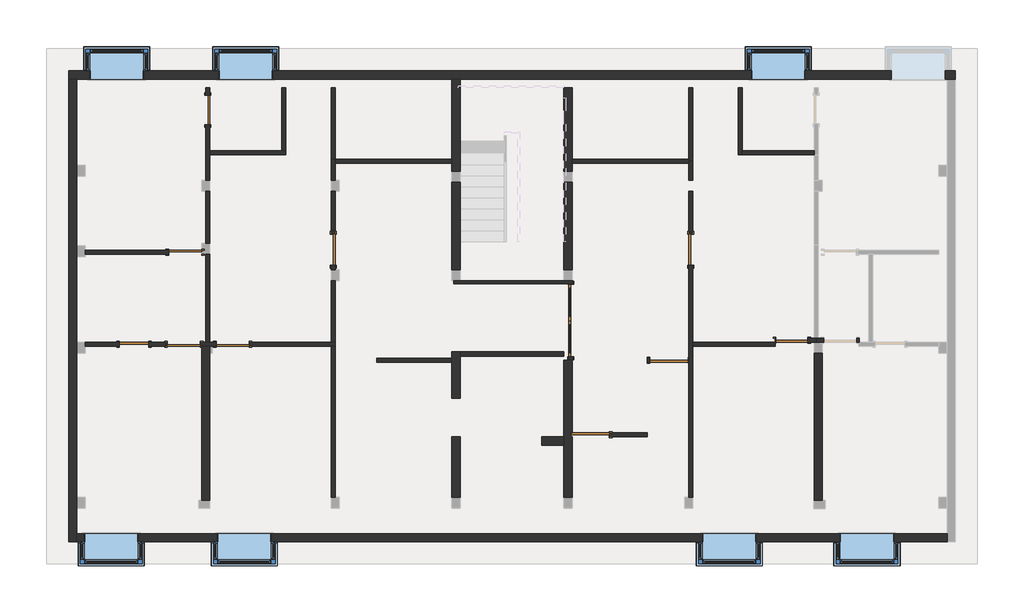
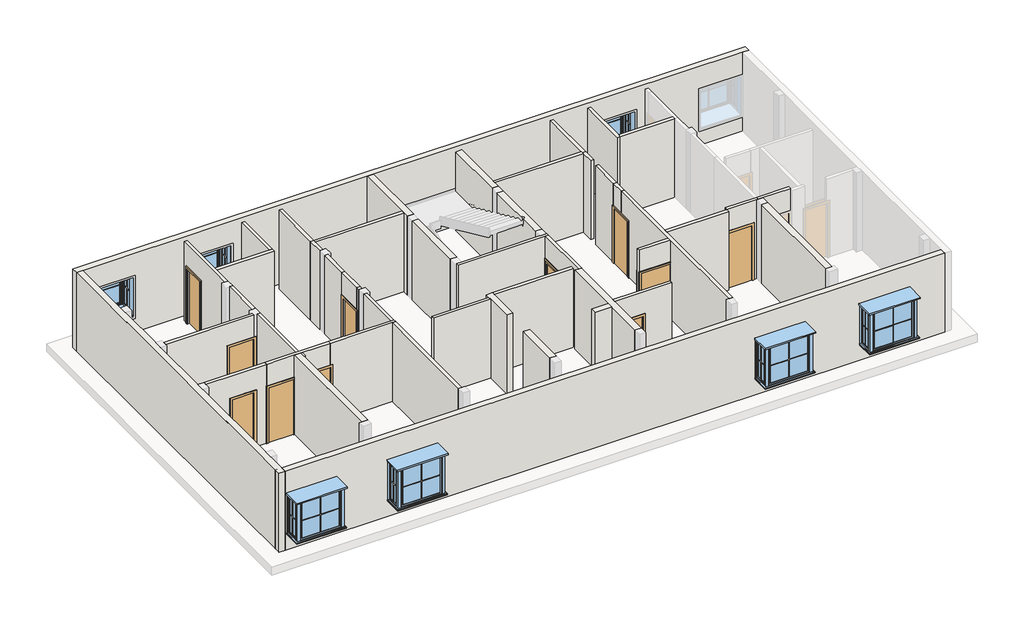
# One storey, part 1 of 2: 48 walls, 11 doors, 7 windows.
"""IFC4 building model written with IfcOpenShell, lengths in millimetres."""

from ifc_helpers import new_model, si_unit, frame, origin, place, context, project, spatial, polyline, outline, extrude, faceted_brep, transform, mapped, element, save
from components import door_04ab2522, m_door_single_panel_05506f71, door_07b5d71c, door_85b31ab1, door_1991e9a2, door_4c0a2014, door_82def9da, m_door_single_panel_3_x7_f8176753, m_door_single_panel_3_x7_ebb67e73, window_19bbd869

model = new_model("IFC4")

# Units and contexts
model_context = context("Model", 3, world=origin())
ifc_project = project(units=[si_unit("LENGTHUNIT", "METRE", prefix="MILLI")], contexts=[model_context])

# Site, building, storey
site = spatial("IfcSite", under=ifc_project)
building = spatial("IfcBuilding", under=site)
storey = spatial("IfcBuildingStorey", under=building, Elevation=16002.0)

# Doors
placement = place(None, origin())
door_shape = door_04ab2522(model_context)
element("IfcDoor", 1, ObjectType="M_Door-Double-Glass : 6'7\"X7'", at=placement, inside=storey, context=model_context, shape_type="MappedRepresentation", body=[
    mapped(door_shape, transform((1217.5394962, 1183.3817656, 16002.0), x_axis=(0.0, 1.0, 0.0), y_axis=(-1.0, 0.0, 0.0), z_axis=(0.0, 0.0, 1.0))),
])
m_door_single_panel_shape = m_door_single_panel_05506f71(model_context)
element("IfcDoor", 2, ObjectType="M_Door-Single-Panel", at=placement, inside=storey, context=model_context, shape_type="MappedRepresentation", body=[
    mapped(m_door_single_panel_shape, transform((1745.3012085, -1975.7432663, 16002.0), x_axis=(-1.0, 0.0, 0.0), y_axis=(0.0, -1.0, 0.0), z_axis=(0.0, 0.0, 1.0))),
])
element("IfcDoor", 3, ObjectType="M_Door-Single-Panel", at=placement, inside=storey, context=model_context, shape_type="MappedRepresentation", body=[
    mapped(m_door_single_panel_shape, transform((3933.4813133, 90.9578621, 16002.0), x_axis=(1.0, 0.0, 0.0), y_axis=(0.0, 1.0, 0.0), z_axis=(0.0, 0.0, 1.0))),
])
door_2_shape = door_07b5d71c(model_context)
element("IfcDoor", 4, ObjectType="M_Door-Single-Panel : 2'10\"X7' 2", at=placement, inside=storey, context=model_context, shape_type="MappedRepresentation", body=[
    mapped(door_2_shape, transform((-5360.3487995, 3142.9626891, 16002.0), x_axis=(0.0, -1.0, 0.0), y_axis=(1.0, 0.0, 0.0), z_axis=(0.0, 0.0, 1.0))),
])
door_3_shape = door_85b31ab1(model_context)
element("IfcDoor", 5, ObjectType="M_Door-Single-Panel : 2'10\"X7' 2", at=placement, inside=storey, context=model_context, shape_type="MappedRepresentation", body=[
    mapped(door_3_shape, transform((4532.9512082, 3142.9626891, 16002.0), x_axis=(0.0, -1.0, 0.0), y_axis=(1.0, 0.0, 0.0), z_axis=(0.0, 0.0, 1.0))),
])
door_4_shape = door_1991e9a2(model_context)
element("IfcDoor", 6, ObjectType="M_Door-Single-Panel : 2'11\"X7' 3", at=placement, inside=storey, context=model_context, shape_type="MappedRepresentation", body=[
    mapped(door_4_shape, transform((7330.1405552, 640.4567334, 16002.0), x_axis=(1.0, 0.0, 0.0), y_axis=(0.0, 1.0, 0.0), z_axis=(0.0, 0.0, 1.0))),
])
door_5_shape = door_4c0a2014(model_context)
element("IfcDoor", 7, ObjectType="M_Door-Single-Panel : 2'8\"X7'", at=placement, inside=storey, context=model_context, shape_type="MappedRepresentation", body=[
    mapped(door_5_shape, transform((-10873.4462614, 526.1567334, 16002.0), x_axis=(1.0, 0.0, 0.0), y_axis=(0.0, 1.0, 0.0), z_axis=(0.0, 0.0, 1.0))),
])
door_6_shape = door_82def9da(model_context)
element("IfcDoor", 8, ObjectType="M_Door-Single-Panel : 2'8\"X7'", at=placement, inside=storey, context=model_context, shape_type="MappedRepresentation", body=[
    mapped(door_6_shape, transform((-8827.4487992, 7008.6751452, 16002.0), x_axis=(0.0, 1.0, 0.0), y_axis=(-1.0, 0.0, 0.0), z_axis=(0.0, 0.0, 1.0))),
])
m_door_single_panel_3_x7_shape = m_door_single_panel_3_x7_f8176753(model_context)
element("IfcDoor", 9, ObjectType="M_Door-Single-Panel : 3'X7'", at=placement, inside=storey, context=model_context, shape_type="MappedRepresentation", body=[
    mapped(m_door_single_panel_3_x7_shape, transform((-9456.0987989, 3078.8567332, 16002.0), x_axis=(1.0, 0.0, 0.0), y_axis=(0.0, 1.0, 0.0), z_axis=(0.0, 0.0, 1.0))),
])
element("IfcDoor", 10, ObjectType="M_Door-Single-Panel : 3'X7'", at=placement, inside=storey, context=model_context, shape_type="MappedRepresentation", body=[
    mapped(m_door_single_panel_3_x7_shape, transform((-8144.8381465, 526.1567334, 16002.0), x_axis=(-1.0, 0.0, 0.0), y_axis=(0.0, -1.0, 0.0), z_axis=(0.0, 0.0, 1.0))),
])
m_door_single_panel_3_x7_2_shape = m_door_single_panel_3_x7_ebb67e73(model_context)
element("IfcDoor", 11, ObjectType="M_Door-Single-Panel : 3'X7'", at=placement, inside=storey, context=model_context, shape_type="MappedRepresentation", body=[
    mapped(m_door_single_panel_3_x7_2_shape, transform((-9494.1987992, 526.1567334, 16002.0), x_axis=(1.0, 0.0, 0.0), y_axis=(0.0, 1.0, 0.0), z_axis=(0.0, 0.0, 1.0))),
])

# Walls
element("IfcWall", 12, ObjectType="3.5\"", at=placement, inside=storey, context=model_context, shape_type="Brep", body=[
    faceted_brep([(-2020.2487998, 2196.2067742, 16002.0), (1158.0082462, 2196.2067742, 16002.0), (1272.3082462, 2196.2067742, 16002.0), (1272.3082462, 2196.2067742, 19050.0), (1158.0082462, 2196.2067742, 19050.0), (-2020.2487998, 2196.2067742, 19050.0), (-2020.2487998, 2285.1067742, 16002.0), (-2020.2487998, 2285.1067742, 19050.0), (-1845.5417538, 2285.1067742, 19050.0), (1024.6582462, 2285.1067742, 19050.0), (1253.2582462, 2285.1067742, 19050.0), (1272.3082462, 2285.1067742, 19050.0), (1272.3082462, 2285.1067742, 16002.0), (1253.2582462, 2285.1067742, 16002.0), (1024.6582462, 2285.1067742, 16002.0), (-1845.5417538, 2285.1067742, 16002.0)], [[[0, 1, 2, 3, 4, 5]], [[6, 7, 8, 9, 10, 11, 12, 13, 14, 15]], [[2, 1, 0, 6, 15, 14, 13, 12]], [[5, 4, 3, 11, 10, 9, 8, 7]], [[0, 5, 7, 6]], [[3, 2, 12, 11]]]),
])
element("IfcWall", 13, ObjectType="4.5\"", at=placement, inside=storey, context=model_context, shape_type="SweptSolid", body=[
    extrude(outline(polyline([(3132.0737955, 19050.0), (3628.3344162, 19050.0), (3628.3344162, 16002.0), (3574.7626891, 16002.0), (3574.7626891, 18135.6), (3132.0737955, 18135.6), (3132.0737955, 19050.0)])), frame((4475.8012082, 0.0, 0.0), z_axis=(1.0, 0.0, 0.0), x_axis=(0.0, 1.0, 0.0)), (0.0, 0.0, 1.0), 114.3),
])
element("IfcWall", 14, ObjectType="4.5\"", at=placement, inside=storey, context=model_context, shape_type="SweptSolid", body=[
    extrude(outline(polyline([(2711.1626891, 19050.0), (3671.8272228, 19050.0), (3671.8272228, 16002.0), (3574.7626891, 16002.0), (3574.7626891, 18135.6), (2711.1626891, 18135.6), (2711.1626891, 19050.0)])), frame((-5417.4987995, 0.0, 0.0), z_axis=(1.0, 0.0, 0.0), x_axis=(0.0, 1.0, 0.0)), (0.0, 0.0, 1.0), 114.3),
])
element("IfcWall", 15, ObjectType="4.5\"", at=placement, inside=storey, context=model_context, shape_type="Brep", body=[
    faceted_brep([(-7690.1644155, 469.0067334, 19050.0), (-8713.148796, 469.0067334, 19050.0), (-8771.750543, 469.0067334, 19050.0), (-9000.350543, 469.0067334, 19050.0), (-10009.8462614, 469.0067334, 19050.0), (-10009.8462614, 469.0067334, 16002.0), (-9951.3987992, 469.0067334, 16002.0), (-9951.3987992, 469.0067334, 18135.6), (-9036.9987992, 469.0067334, 18135.6), (-9036.9987992, 469.0067334, 16002.0), (-9000.350543, 469.0067334, 16002.0), (-8771.750543, 469.0067334, 16002.0), (-8713.148796, 469.0067334, 16002.0), (-8602.0381465, 469.0067334, 16002.0), (-8602.0381465, 469.0067334, 18135.6), (-7690.1644155, 469.0067334, 18135.6), (-10009.8462614, 583.3067334, 19050.0), (-7690.1644155, 583.3067334, 19050.0), (-7690.1644155, 583.3067334, 18135.6), (-8602.0381465, 583.3067334, 18135.6), (-8602.0381465, 583.3067334, 16002.0), (-9036.9987992, 583.3067334, 16002.0), (-9036.9987992, 583.3067334, 18135.6), (-9951.3987992, 583.3067334, 18135.6), (-9951.3987992, 583.3067334, 16002.0), (-10009.8462614, 583.3067334, 16002.0)], [[[0, 1, 2, 3, 4, 5, 6, 7, 8, 9, 10, 11, 12, 13, 14, 15]], [[16, 17, 18, 19, 20, 21, 22, 23, 24, 25]], [[5, 25, 24, 6]], [[9, 21, 20, 13, 12, 11, 10]], [[17, 0, 15, 18]], [[4, 3, 2, 1, 0, 17, 16]], [[5, 4, 16, 25]], [[8, 22, 21, 9]], [[7, 23, 22, 8]], [[23, 7, 6, 24]], [[19, 14, 13, 20]], [[14, 19, 18, 15]]]),
])
element("IfcWall", 16, ObjectType="4.5\"", at=placement, inside=storey, context=model_context, shape_type="Brep", body=[
    faceted_brep([(8000.0512079, 583.3067334, 16002.0), (8000.0512079, 583.3067334, 19050.0), (7942.9012047, 583.3067334, 19050.0), (6862.7668241, 583.3067334, 19050.0), (6862.7668241, 583.3067334, 16002.0), (6885.6405552, 583.3067334, 16002.0), (6885.6405552, 583.3067334, 18135.6), (7774.6405552, 583.3067334, 18135.6), (7774.6405552, 583.3067334, 16002.0), (7942.9012047, 583.3067334, 16002.0), (8000.0512079, 697.6067334, 19050.0), (8000.0512079, 697.6067334, 16002.0), (7942.9012079, 697.6067334, 16002.0), (7774.6405552, 697.6067334, 16002.0), (7774.6405552, 697.6067334, 18135.6), (6885.6405552, 697.6067334, 18135.6), (6885.6405552, 697.6067334, 16002.0), (6862.7668241, 697.6067334, 16002.0), (6862.7668241, 697.6067334, 19050.0), (7942.9012079, 697.6067334, 19050.0)], [[[0, 1, 2, 3, 4, 5, 6, 7, 8, 9]], [[10, 11, 12, 13, 14, 15, 16, 17, 18, 19]], [[4, 17, 16, 5]], [[11, 0, 9, 8, 13, 12]], [[1, 0, 11, 10]], [[3, 2, 1, 10, 19, 18]], [[4, 3, 18, 17]], [[7, 14, 13, 8]], [[14, 7, 6, 15]], [[15, 6, 5, 16]]]),
])
element("IfcWall", 17, ObjectType="4.5\"", at=placement, inside=storey, context=model_context, shape_type="Brep", body=[
    faceted_brep([(9187.5012047, 583.3067334, 16002.0), (9187.5012047, 583.3067334, 19050.0), (8171.5012047, 583.3067334, 19050.0), (8000.0512079, 583.3067334, 19050.0), (8000.0512079, 583.3067334, 16002.0), (8171.5012047, 583.3067334, 16002.0), (8209.6012079, 583.3067334, 16002.0), (8209.6012079, 583.3067334, 18135.6), (9124.0012079, 583.3067334, 18135.6), (9124.0012079, 583.3067334, 16002.0), (9187.5012047, 697.6067334, 19050.0), (9187.5012047, 697.6067334, 16002.0), (9124.0012079, 697.6067334, 16002.0), (9124.0012079, 697.6067334, 18135.6), (8209.6012079, 697.6067334, 18135.6), (8209.6012079, 697.6067334, 16002.0), (8057.2012079, 697.6067334, 16002.0), (8000.0512079, 697.6067334, 16002.0), (8000.0512079, 697.6067334, 19050.0), (8057.2012079, 697.6067334, 19050.0)], [[[0, 1, 2, 3, 4, 5, 6, 7, 8, 9]], [[10, 11, 12, 13, 14, 15, 16, 17, 18, 19]], [[11, 0, 9, 12]], [[4, 17, 16, 15, 6, 5]], [[1, 0, 11, 10]], [[3, 2, 1, 10, 19, 18]], [[4, 3, 18, 17]], [[7, 14, 13, 8]], [[8, 13, 12, 9]], [[14, 7, 6, 15]]]),
])
element("IfcWall", 18, ObjectType="4.5\"", at=placement, inside=storey, context=model_context, shape_type="SweptSolid", body=[
    extrude(outline(polyline([(16002.0, 3334.0114184), (19050.0, 3334.0114184), (19050.0, 1250.0012085), (18135.6, 1250.0012085), (18135.6, 2278.7012085), (16002.0, 2278.7012085), (16002.0, 3334.0114184)])), frame((0.0, -2032.8932663, 0.0), z_axis=(0.0, 1.0, 0.0), x_axis=(0.0, 0.0, 1.0)), (0.0, 0.0, 1.0), 114.3),
])
element("IfcWall", 19, ObjectType="4.5\"", at=placement, inside=storey, context=model_context, shape_type="SweptSolid", body=[
    extrude(outline(polyline([(18135.6, 4466.8813133), (16002.0, 4466.8813133), (16002.0, 4475.8012082), (19050.0, 4475.8012082), (19050.0, 3334.0114184), (16002.0, 3334.0114184), (16002.0, 3400.0813133), (18135.6, 3400.0813133), (18135.6, 4466.8813133)])), frame((0.0, 33.8078621, 0.0), z_axis=(0.0, 1.0, 0.0), x_axis=(0.0, 0.0, 1.0)), (0.0, 0.0, 1.0), 114.3),
])
element("IfcWall", 20, ObjectType="4.5\"", at=placement, inside=storey, context=model_context, shape_type="SweptSolid", body=[
    extrude(outline(polyline([(1021.4012085, 202.3067742), (-1848.7987998, 202.3067742), (-1848.7987998, 316.6067742), (1021.4012085, 316.6067742), (1021.4012085, 202.3067742)])), frame((0.0, 0.0, 16002.0), z_axis=(0.0, 0.0, 1.0), x_axis=(1.0, 0.0, 0.0)), (0.0, 0.0, 1.0), 3048.0),
])
element("IfcWall", 21, ObjectType="4.5\"", at=placement, inside=storey, context=model_context, shape_type="Brep", body=[
    faceted_brep([(1158.0082462, 2196.2067742, 16002.0), (1158.0082462, 2186.6817656, 16002.0), (1158.0082462, 2186.6817656, 18135.6), (1158.0082462, 180.0817656, 18135.6), (1158.0082462, 180.0817656, 16002.0), (1158.0082462, 90.9578621, 16002.0), (1158.0082462, 90.9578621, 19050.0), (1158.0082462, 2196.2067742, 19050.0), (1272.3082462, 2186.6817656, 18135.6), (1272.3082462, 2186.6817656, 16002.0), (1272.3082462, 2196.2067742, 16002.0), (1272.3082462, 2196.2067742, 19050.0), (1272.3082462, 90.9578621, 19050.0), (1272.3082462, 90.9578621, 16002.0), (1272.3082462, 180.0817656, 16002.0), (1272.3082462, 180.0817656, 18135.6), (1250.0012085, 90.9578621, 16002.0), (1250.0012085, 90.9578621, 19050.0)], [[[0, 1, 2, 3, 4, 5, 6, 7]], [[8, 9, 10, 11, 12, 13, 14, 15]], [[14, 13, 16, 5, 4]], [[10, 9, 1, 0]], [[6, 5, 16, 13, 12, 17]], [[7, 6, 17, 12, 11]], [[0, 7, 11, 10]], [[2, 1, 9, 8]], [[3, 2, 8, 15]], [[4, 3, 15, 14]]]),
])
element("IfcWall", 22, ObjectType="4.5\"", at=placement, inside=storey, context=model_context, shape_type="Brep", body=[
    faceted_brep([(1250.0012085, 5536.3067329, 16002.0), (4475.8012082, 5536.3067329, 16002.0), (4475.8012082, 5536.3067329, 19050.0), (1250.0012085, 5536.3067329, 19050.0), (1250.0012085, 5650.6067329, 16002.0), (1250.0012085, 5650.6067329, 19050.0), (4475.8012082, 5650.6067329, 19050.0), (4475.8012082, 5650.6067329, 16002.0), (4475.8012082, 5593.4567329, 16002.0), (4475.8012082, 5593.4567329, 19050.0)], [[[0, 1, 2, 3]], [[4, 5, 6, 7]], [[1, 0, 4, 7, 8]], [[3, 2, 9, 6, 5]], [[2, 1, 8, 7, 6, 9]], [[0, 3, 5, 4]]]),
])
element("IfcWall", 23, ObjectType="4.5\"", at=placement, inside=storey, context=model_context, shape_type="SweptSolid", body=[
    extrude(outline(polyline([(-5417.4987995, -3709.2932193), (-5417.4987995, 469.0067334), (-5303.1987995, 469.0067334), (-5303.1987995, -3709.2932193), (-5417.4987995, -3709.2932193)])), frame((0.0, 0.0, 16002.0), z_axis=(0.0, 0.0, 1.0), x_axis=(1.0, 0.0, 0.0)), (0.0, 0.0, 1.0), 3048.0),
])
element("IfcWall", 24, ObjectType="4.5\" 2", at=placement, inside=storey, context=model_context, shape_type="SweptSolid", body=[
    extrude(outline(polyline([(19050.0, -8998.8987989), (19050.0, -12224.6987989), (16002.0, -12224.6987989), (16002.0, -9913.2987989), (18135.6, -9913.2987989), (18135.6, -8998.8987989), (19050.0, -8998.8987989)])), frame((0.0, 3021.7067332, 0.0), z_axis=(0.0, 1.0, 0.0), x_axis=(0.0, 0.0, 1.0)), (0.0, 0.0, 1.0), 114.3),
])
element("IfcWall", 25, ObjectType="4.5\" 2", at=placement, inside=storey, context=model_context, shape_type="SweptSolid", body=[
    extrude(outline(polyline([(-8770.2987992, 4761.606733), (-8770.2987992, 3326.5067332), (-8884.5987992, 3326.5067332), (-8884.5987992, 4761.606733), (-8770.2987992, 4761.606733)])), frame((0.0, 0.0, 16002.0), z_axis=(0.0, 0.0, 1.0), x_axis=(1.0, 0.0, 0.0)), (0.0, 0.0, 1.0), 3048.0),
])
element("IfcWall", 26, ObjectType="4.5\" 2", at=placement, inside=storey, context=model_context, shape_type="Brep", body=[
    faceted_brep([(-8770.2987992, 7415.0751452, 18135.6), (-8770.2987992, 7415.0751452, 16002.0), (-8770.2987992, 7631.8067329, 16002.0), (-8770.2987992, 7631.8067329, 19050.0), (-8770.2987992, 5879.2067329, 19050.0), (-8770.2987992, 5764.9067329, 19050.0), (-8770.2987992, 5066.406733, 19050.0), (-8770.2987992, 5066.406733, 16002.0), (-8770.2987992, 5764.9067329, 16002.0), (-8770.2987992, 5879.2067329, 16002.0), (-8770.2987992, 6602.2751452, 16002.0), (-8770.2987992, 6602.2751452, 18135.6), (-8884.5987992, 7631.8067329, 16002.0), (-8884.5987992, 7415.0751452, 16002.0), (-8884.5987992, 7415.0751452, 18135.6), (-8884.5987992, 6602.2751452, 18135.6), (-8884.5987992, 6602.2751452, 16002.0), (-8884.5987992, 5066.406733, 16002.0), (-8884.5987992, 5066.406733, 19050.0), (-8884.5987992, 7631.8067329, 19050.0)], [[[0, 1, 2, 3, 4, 5, 6, 7, 8, 9, 10, 11]], [[12, 13, 14, 15, 16, 17, 18, 19]], [[2, 1, 13, 12]], [[10, 9, 8, 7, 17, 16]], [[3, 2, 12, 19]], [[6, 5, 4, 3, 19, 18]], [[7, 6, 18, 17]], [[14, 13, 1, 0]], [[15, 14, 0, 11]], [[16, 15, 11, 10]]]),
])
element("IfcWall", 27, ObjectType="4.5\" 2", at=placement, inside=storey, context=model_context, shape_type="Brep", body=[
    faceted_brep([(-8770.2987992, 5764.9067329, 16002.0), (-6674.7987994, 5764.9067329, 16002.0), (-6674.7987994, 5764.9067329, 19050.0), (-8770.2987992, 5764.9067329, 19050.0), (-8770.2987992, 5879.2067329, 16002.0), (-8770.2987992, 5879.2067329, 19050.0), (-6789.0987994, 5879.2067329, 19050.0), (-6674.7987994, 5879.2067329, 19050.0), (-6674.7987994, 5879.2067329, 16002.0), (-6789.0987994, 5879.2067329, 16002.0)], [[[0, 1, 2, 3]], [[4, 5, 6, 7, 8, 9]], [[1, 0, 4, 9, 8]], [[3, 2, 7, 6, 5]], [[0, 3, 5, 4]], [[2, 1, 8, 7]]]),
])
element("IfcWall", 28, ObjectType="4.5\" 2", at=placement, inside=storey, context=model_context, shape_type="SweptSolid", body=[
    extrude(outline(polyline([(-6674.7987994, 7631.8067329), (-6674.7987994, 5879.2067329), (-6789.0987994, 5879.2067329), (-6789.0987994, 7631.8067329), (-6674.7987994, 7631.8067329)])), frame((0.0, 0.0, 16002.0), z_axis=(0.0, 0.0, 1.0), x_axis=(1.0, 0.0, 0.0)), (0.0, 0.0, 1.0), 3048.0),
])
element("IfcWall", 29, ObjectType="4.5\" 2", at=placement, inside=storey, context=model_context, shape_type="SweptSolid", body=[
    extrude(outline(polyline([(18135.6, -10467.0462614), (16002.0, -10467.0462614), (16002.0, -10009.8462614), (19050.0, -10009.8462614), (19050.0, -12224.6987989), (16002.0, -12224.6987989), (16002.0, -11279.8462614), (18135.6, -11279.8462614), (18135.6, -10467.0462614)])), frame((0.0, 469.0067334, 0.0), z_axis=(0.0, 1.0, 0.0), x_axis=(0.0, 0.0, 1.0)), (0.0, 0.0, 1.0), 114.3),
])
element("IfcWall", 30, ObjectType="4.5\" 2", at=placement, inside=storey, context=model_context, shape_type="SweptSolid", body=[
    extrude(outline(polyline([(-8770.298796, 3021.7067332), (-8770.298796, 583.3067804), (-8884.598796, 583.3067804), (-8884.598796, 3021.7067332), (-8770.298796, 3021.7067332)])), frame((0.0, 0.0, 16002.0), z_axis=(0.0, 0.0, 1.0), x_axis=(1.0, 0.0, 0.0)), (0.0, 0.0, 1.0), 3048.0),
])
element("IfcWall", 31, ObjectType="4.5\" 2", at=placement, inside=storey, context=model_context, shape_type="Brep", body=[
    faceted_brep([(-5303.1987995, 469.0067334, 19050.0), (-5417.4987995, 469.0067334, 19050.0), (-7690.1644155, 469.0067334, 19050.0), (-7690.1644155, 469.0067334, 18135.6), (-7687.6381465, 469.0067334, 18135.6), (-7687.6381465, 469.0067334, 16002.0), (-5417.4987995, 469.0067334, 16002.0), (-5303.1987995, 469.0067334, 16002.0), (-7690.1644155, 583.3067334, 19050.0), (-5417.4987995, 583.3067334, 19050.0), (-5303.1987995, 583.3067334, 19050.0), (-5303.1987995, 583.3067334, 16002.0), (-5417.4987995, 583.3067334, 16002.0), (-7687.6381465, 583.3067334, 16002.0), (-7687.6381465, 583.3067334, 18135.6), (-7690.1644155, 583.3067334, 18135.6)], [[[0, 1, 2, 3, 4, 5, 6, 7]], [[8, 9, 10, 11, 12, 13, 14, 15]], [[11, 7, 6, 5, 13, 12]], [[2, 1, 0, 10, 9, 8]], [[2, 8, 15, 3]], [[0, 7, 11, 10]], [[14, 4, 3, 15]], [[4, 14, 13, 5]]]),
])
element("IfcWall", 32, ObjectType="4.5\" 2", at=placement, inside=storey, context=model_context, shape_type="SweptSolid", body=[
    extrude(outline(polyline([(-5303.1987995, 2285.1067802), (-5303.1987995, 583.3067334), (-5417.4987995, 583.3067334), (-5417.4987995, 2285.1067802), (-5303.1987995, 2285.1067802)])), frame((0.0, 0.0, 16002.0), z_axis=(0.0, 0.0, 1.0), x_axis=(1.0, 0.0, 0.0)), (0.0, 0.0, 1.0), 3048.0),
])
element("IfcWall", 33, ObjectType="4.5\" 2", at=placement, inside=storey, context=model_context, shape_type="Brep", body=[
    faceted_brep([(-5303.1987995, 2589.9067802, 16002.0), (-5303.1987995, 2711.1626891, 16002.0), (-5303.1987995, 2711.1626891, 18135.6), (-5303.1987995, 2711.1626891, 19050.0), (-5303.1987995, 2589.9067802, 19050.0), (-5417.4987995, 2589.9067802, 16002.0), (-5417.4987995, 2589.9067802, 19050.0), (-5417.4987995, 2711.1626891, 19050.0), (-5417.4987995, 2711.1626891, 18135.6), (-5417.4987995, 2711.1626891, 16002.0)], [[[0, 1, 2, 3, 4]], [[5, 6, 7, 8, 9]], [[1, 0, 5, 9]], [[3, 2, 1, 9, 8, 7]], [[4, 3, 7, 6]], [[0, 4, 6, 5]]]),
])
element("IfcWall", 34, ObjectType="4.5\" 2", at=placement, inside=storey, context=model_context, shape_type="SweptSolid", body=[
    extrude(outline(polyline([(-5303.1987995, 4761.606733), (-5303.1987995, 3671.8272228), (-5417.4987995, 3671.8272228), (-5417.4987995, 4761.606733), (-5303.1987995, 4761.606733)])), frame((0.0, 0.0, 16002.0), z_axis=(0.0, 0.0, 1.0), x_axis=(1.0, 0.0, 0.0)), (0.0, 0.0, 1.0), 3048.0),
])
element("IfcWall", 35, ObjectType="4.5\" 2", at=placement, inside=storey, context=model_context, shape_type="Brep", body=[
    faceted_brep([(-5303.1987995, 5066.406733, 16002.0), (-5303.1987995, 5536.3067329, 16002.0), (-5303.1987995, 5650.6067329, 16002.0), (-5303.1987995, 5650.6067329, 19050.0), (-5303.1987995, 5536.3067329, 19050.0), (-5303.1987995, 5066.406733, 19050.0), (-5417.4987995, 5066.406733, 16002.0), (-5417.4987995, 5066.406733, 19050.0), (-5417.4987995, 5650.6067329, 19050.0), (-5417.4987995, 5650.6067329, 16002.0)], [[[0, 1, 2, 3, 4, 5]], [[6, 7, 8, 9]], [[2, 1, 0, 6, 9]], [[5, 4, 3, 8, 7]], [[0, 5, 7, 6]], [[3, 2, 9, 8]]]),
])
element("IfcWall", 36, ObjectType="4.5\" 2", at=placement, inside=storey, context=model_context, shape_type="SweptSolid", body=[
    extrude(outline(polyline([(-2077.3987998, 5536.3067329), (-5303.1987995, 5536.3067329), (-5303.1987995, 5650.6067329), (-2077.3987998, 5650.6067329), (-2077.3987998, 5536.3067329)])), frame((0.0, 0.0, 16002.0), z_axis=(0.0, 0.0, 1.0), x_axis=(1.0, 0.0, 0.0)), (0.0, 0.0, 1.0), 3048.0),
])
element("IfcWall", 37, ObjectType="4.5\" 2", at=placement, inside=storey, context=model_context, shape_type="SweptSolid", body=[
    extrude(outline(polyline([(-5417.4987995, 5650.6067329), (-5417.4987995, 7631.8067329), (-5303.1987995, 7631.8067329), (-5303.1987995, 5650.6067329), (-5417.4987995, 5650.6067329)])), frame((0.0, 0.0, 16002.0), z_axis=(0.0, 0.0, 1.0), x_axis=(1.0, 0.0, 0.0)), (0.0, 0.0, 1.0), 3048.0),
])
element("IfcWall", 38, ObjectType="4.5\" 2", at=placement, inside=storey, context=model_context, shape_type="Brep", body=[
    faceted_brep([(4475.8012082, 5593.4567329, 16002.0), (4475.8012082, 5536.3067329, 16002.0), (4475.8012082, 5066.40678, 16002.0), (4475.8012082, 5066.40678, 19050.0), (4475.8012082, 5536.3067329, 19050.0), (4475.8012082, 5593.4567329, 19050.0), (4590.1012082, 5593.4567329, 16002.0), (4590.1012082, 5593.4567329, 19050.0), (4590.1012082, 5066.40678, 19050.0), (4590.1012082, 5066.40678, 16002.0)], [[[0, 1, 2, 3, 4, 5]], [[6, 7, 8, 9]], [[2, 1, 0, 6, 9]], [[3, 2, 9, 8]], [[5, 4, 3, 8, 7]], [[0, 5, 7, 6]]]),
])
element("IfcWall", 39, ObjectType="4.5\" 2", at=placement, inside=storey, context=model_context, shape_type="SweptSolid", body=[
    extrude(outline(polyline([(4475.8012082, 3628.3344162), (4475.8012082, 4761.606733), (4590.1012082, 4761.606733), (4590.1012082, 3628.3344162), (4475.8012082, 3628.3344162)])), frame((0.0, 0.0, 16002.0), z_axis=(0.0, 0.0, 1.0), x_axis=(1.0, 0.0, 0.0)), (0.0, 0.0, 1.0), 3048.0),
])
element("IfcWall", 40, ObjectType="4.5\" 2", at=placement, inside=storey, context=model_context, shape_type="Brep", body=[
    faceted_brep([(4475.8012082, -3709.2932193, 16002.0), (4475.8012082, -3709.2932193, 19050.0), (4475.8012082, 33.8078621, 19050.0), (4475.8012082, 148.1078621, 19050.0), (4475.8012082, 3132.0737955, 19050.0), (4475.8012082, 3132.0737955, 18135.6), (4475.8012082, 2711.1626891, 18135.6), (4475.8012082, 2711.1626891, 16002.0), (4475.8012082, 148.1078621, 16002.0), (4475.8012082, 33.8078621, 16002.0), (4590.1012082, -3709.2932193, 19050.0), (4590.1012082, -3709.2932193, 16002.0), (4590.1012082, 469.0067334, 16002.0), (4590.1012082, 583.3067334, 16002.0), (4590.1012082, 2711.1626891, 16002.0), (4590.1012082, 2711.1626891, 18135.6), (4590.1012082, 3132.0737955, 18135.6), (4590.1012082, 3132.0737955, 19050.0), (4590.1012082, 583.3067334, 19050.0), (4590.1012082, 469.0067334, 19050.0)], [[[0, 1, 2, 3, 4, 5, 6, 7, 8, 9]], [[10, 11, 12, 13, 14, 15, 16, 17, 18, 19]], [[11, 0, 9, 8, 7, 14, 13, 12]], [[1, 0, 11, 10]], [[4, 3, 2, 1, 10, 19, 18, 17]], [[4, 17, 16, 5]], [[6, 15, 14, 7]], [[15, 6, 5, 16]]]),
])
element("IfcWall", 41, ObjectType="4.5\" 2", at=placement, inside=storey, context=model_context, shape_type="SweptSolid", body=[
    extrude(outline(polyline([(6862.7668241, 469.0067334), (4590.1012082, 469.0067334), (4590.1012082, 583.3067334), (6862.7668241, 583.3067334), (6862.7668241, 469.0067334)])), frame((0.0, 0.0, 16002.0), z_axis=(0.0, 0.0, 1.0), x_axis=(1.0, 0.0, 0.0)), (0.0, 0.0, 1.0), 3048.0),
])
element("IfcWall", 42, ObjectType="4.5\" 2", at=placement, inside=storey, context=model_context, shape_type="Brep", body=[
    faceted_brep([(4590.1012082, 5593.4567329, 16002.0), (4590.1012082, 7631.8067329, 16002.0), (4590.1012082, 7631.8067329, 19050.0), (4590.1012082, 5593.4567329, 19050.0), (4475.8012082, 5593.4567329, 16002.0), (4475.8012082, 5593.4567329, 19050.0), (4475.8012082, 5650.6067329, 19050.0), (4475.8012082, 7631.8067329, 19050.0), (4475.8012082, 7631.8067329, 16002.0), (4475.8012082, 5650.6067329, 16002.0)], [[[0, 1, 2, 3]], [[4, 5, 6, 7, 8, 9]], [[1, 0, 4, 9, 8]], [[2, 1, 8, 7]], [[3, 2, 7, 6, 5]], [[0, 3, 5, 4]]]),
])
element("IfcWall", 43, ObjectType="4.5\" 2", at=placement, inside=storey, context=model_context, shape_type="Brep", body=[
    faceted_brep([(5847.401208, 7631.8067329, 16002.0), (5847.401208, 5764.9067329, 16002.0), (5847.401208, 5764.9067329, 19050.0), (5847.401208, 7631.8067329, 19050.0), (5961.701208, 7631.8067329, 16002.0), (5961.701208, 7631.8067329, 19050.0), (5961.701208, 5879.2067329, 19050.0), (5961.701208, 5764.9067329, 19050.0), (5961.701208, 5764.9067329, 16002.0), (5961.701208, 5879.2067329, 16002.0)], [[[0, 1, 2, 3]], [[4, 5, 6, 7, 8, 9]], [[1, 0, 4, 9, 8]], [[3, 2, 7, 6, 5]], [[0, 3, 5, 4]], [[2, 1, 8, 7]]]),
])
element("IfcWall", 44, ObjectType="4.5\" 2", at=placement, inside=storey, context=model_context, shape_type="SweptSolid", body=[
    extrude(outline(polyline([(7942.9012079, 5764.9067329), (5961.701208, 5764.9067329), (5961.701208, 5879.2067329), (7942.9012079, 5879.2067329), (7942.9012079, 5764.9067329)])), frame((0.0, 0.0, 16002.0), z_axis=(0.0, 0.0, 1.0), x_axis=(1.0, 0.0, 0.0)), (0.0, 0.0, 1.0), 3048.0),
])
element("IfcWall", 45, ObjectType="4.5\" 2", at=placement, inside=storey, context=model_context, shape_type="SweptSolid", body=[
    extrude(outline(polyline([(-2077.3987998, 33.8078621), (-4161.4090098, 33.8078621), (-4161.4090098, 148.1078621), (-2077.3987998, 148.1078621), (-2077.3987998, 33.8078621)])), frame((0.0, 0.0, 16002.0), z_axis=(0.0, 0.0, 1.0), x_axis=(1.0, 0.0, 0.0)), (0.0, 0.0, 1.0), 3048.0),
])
element("IfcWall", 46, ObjectType="9\"", at=placement, inside=storey, context=model_context, shape_type="Brep", body=[
    faceted_brep([(-12681.8987957, 7860.4067329, 16002.0), (-12453.2987957, 7860.4067329, 16002.0), (-2074.1417538, 7860.4067329, 16002.0), (-1845.5417538, 7860.4067329, 16002.0), (11625.9012075, 7860.4067329, 16002.0), (11854.5012075, 7860.4067329, 16002.0), (11854.5012075, 7860.4067329, 19050.0), (11625.9012075, 7860.4067329, 19050.0), (-1845.5417538, 7860.4067329, 19050.0), (-2074.1417538, 7860.4067329, 19050.0), (-12453.2987957, 7860.4067329, 19050.0), (-12681.8987957, 7860.4067329, 19050.0), (11575.8012075, 7860.4067329, 18152.8), (11575.8012075, 7860.4067329, 16602.0), (10075.8012075, 7860.4067329, 16602.0), (10075.8012075, 7860.4067329, 18152.8), (7702.301208, 7860.4067329, 18152.8), (7702.301208, 7860.4067329, 16602.0), (6202.301208, 7860.4067329, 16602.0), (6202.301208, 7860.4067329, 18152.8), (-7029.6987993, 7860.4067329, 18152.8), (-7029.6987993, 7860.4067329, 16602.0), (-8529.6987993, 7860.4067329, 16602.0), (-8529.6987993, 7860.4067329, 18152.8), (-10598.3987957, 7860.4067329, 18152.8), (-10598.3987957, 7860.4067329, 16602.0), (-12098.3987957, 7860.4067329, 16602.0), (-12098.3987957, 7860.4067329, 18152.8), (-12681.8987957, 8089.0067329, 16002.0), (-12681.8987957, 8089.0067329, 19050.0), (11854.5012075, 8089.0067329, 19050.0), (11854.5012075, 8089.0067329, 16002.0), (11575.8012075, 8089.0067329, 18152.8), (10075.8012075, 8089.0067329, 18152.8), (10075.8012075, 8089.0067329, 16602.0), (11575.8012075, 8089.0067329, 16602.0), (7702.301208, 8089.0067329, 18152.8), (6202.301208, 8089.0067329, 18152.8), (6202.301208, 8089.0067329, 16602.0), (7702.301208, 8089.0067329, 16602.0), (-7029.6987993, 8089.0067329, 18152.8), (-8529.6987993, 8089.0067329, 18152.8), (-8529.6987993, 8089.0067329, 16602.0), (-7029.6987993, 8089.0067329, 16602.0), (-10598.3987957, 8089.0067329, 18152.8), (-12098.3987957, 8089.0067329, 18152.8), (-12098.3987957, 8089.0067329, 16602.0), (-10598.3987957, 8089.0067329, 16602.0)], [[[0, 1, 2, 3, 4, 5, 6, 7, 8, 9, 10, 11], [12, 13, 14, 15], [16, 17, 18, 19], [20, 21, 22, 23], [24, 25, 26, 27]], [[28, 29, 30, 31], [32, 33, 34, 35], [36, 37, 38, 39], [40, 41, 42, 43], [44, 45, 46, 47]], [[5, 4, 3, 2, 1, 0, 28, 31]], [[11, 10, 9, 8, 7, 6, 30, 29]], [[6, 5, 31, 30]], [[0, 11, 29, 28]], [[13, 12, 32, 35]], [[14, 13, 35, 34]], [[15, 14, 34, 33]], [[12, 15, 33, 32]], [[17, 16, 36, 39]], [[18, 17, 39, 38]], [[19, 18, 38, 37]], [[16, 19, 37, 36]], [[21, 20, 40, 43]], [[22, 21, 43, 42]], [[23, 22, 42, 41]], [[20, 23, 41, 40]], [[25, 24, 44, 47]], [[26, 25, 47, 46]], [[27, 26, 46, 45]], [[24, 27, 45, 44]]]),
])
element("IfcWall", 47, ObjectType="9\"", at=placement, inside=storey, context=model_context, shape_type="Brep", body=[
    faceted_brep([(-12453.2987957, -4941.1932661, 16002.0), (-12453.2987957, -4712.5932661, 16002.0), (-12453.2987957, -4014.0932671, 16002.0), (-12453.2987957, -3709.2932671, 16002.0), (-12453.2987957, 278.5067334, 16002.0), (-12453.2987957, 583.3067334, 16002.0), (-12453.2987957, 2951.8567332, 16002.0), (-12453.2987957, 3256.6567332, 16002.0), (-12453.2987957, 5174.3567339, 16002.0), (-12453.2987957, 5479.1567339, 16002.0), (-12453.2987957, 7860.4067329, 16002.0), (-12453.2987957, 7860.4067329, 19050.0), (-12453.2987957, 5479.1567339, 19050.0), (-12453.2987957, 5174.3567339, 19050.0), (-12453.2987957, 3256.6567332, 19050.0), (-12453.2987957, 2951.8567332, 19050.0), (-12453.2987957, 583.3067334, 19050.0), (-12453.2987957, 278.5067334, 19050.0), (-12453.2987957, -3709.2932671, 19050.0), (-12453.2987957, -4014.0932671, 19050.0), (-12453.2987957, -4712.5932661, 19050.0), (-12453.2987957, -4941.1932661, 19050.0), (-12681.8987957, -4941.1932661, 16002.0), (-12681.8987957, -4941.1932661, 19050.0), (-12681.8987957, 7860.4067329, 19050.0), (-12681.8987957, 7860.4067329, 16002.0)], [[[0, 1, 2, 3, 4, 5, 6, 7, 8, 9, 10, 11, 12, 13, 14, 15, 16, 17, 18, 19, 20, 21]], [[22, 23, 24, 25]], [[10, 9, 8, 7, 6, 5, 4, 3, 2, 1, 0, 22, 25]], [[21, 20, 19, 18, 17, 16, 15, 14, 13, 12, 11, 24, 23]], [[11, 10, 25, 24]], [[0, 21, 23, 22]]]),
])
element("IfcWall", 48, ObjectType="9\"", at=placement, inside=storey, context=model_context, shape_type="Brep", body=[
    faceted_brep([(-12453.2987957, -4712.5932661, 16002.0), (-12453.2987957, -4014.0932671, 16002.0), (-12453.2987957, -3709.2932671, 16002.0), (-12453.2987957, 278.5067334, 16002.0), (-12453.2987957, 583.3067334, 16002.0), (-12453.2987957, 2951.8567332, 16002.0), (-12453.2987957, 3256.6567332, 16002.0), (-12453.2987957, 5174.3567339, 16002.0), (-12453.2987957, 5479.1567339, 16002.0), (-12453.2987957, 7860.4067329, 16002.0), (-12453.2987957, 7860.4067329, 19050.0), (-12453.2987957, 5479.1567339, 19050.0), (-12453.2987957, 5174.3567339, 19050.0), (-12453.2987957, 3256.6567332, 19050.0), (-12453.2987957, 2951.8567332, 19050.0), (-12453.2987957, 583.3067334, 19050.0), (-12453.2987957, 278.5067334, 19050.0), (-12453.2987957, -3709.2932671, 19050.0), (-12453.2987957, -4014.0932671, 19050.0), (-12453.2987957, -4712.5932661, 19050.0), (-12681.8987957, -4712.5932661, 16002.0), (-12681.8987957, -4712.5932661, 19050.0), (-12681.8987957, 7860.4067329, 19050.0), (-12681.8987957, 7860.4067329, 16002.0)], [[[0, 1, 2, 3, 4, 5, 6, 7, 8, 9, 10, 11, 12, 13, 14, 15, 16, 17, 18, 19]], [[20, 21, 22, 23]], [[9, 8, 7, 6, 5, 4, 3, 2, 1, 0, 20, 23]], [[19, 18, 17, 16, 15, 14, 13, 12, 11, 10, 22, 21]], [[10, 9, 23, 22]], [[0, 19, 21, 20]]]),
])
element("IfcWall", 49, ObjectType="9\"", at=placement, inside=storey, context=model_context, shape_type="Brep", body=[
    faceted_brep([(-9000.350543, 469.0067334, 16002.0), (-9000.350543, -3785.4932196, 16002.0), (-9000.350543, -3785.4932196, 19050.0), (-9000.350543, 469.0067334, 19050.0), (-8771.750543, 469.0067334, 16002.0), (-8771.750543, 469.0067334, 19050.0), (-8771.750543, 278.5067334, 19050.0), (-8771.750543, -3785.4932196, 19050.0), (-8771.750543, -3785.4932196, 16002.0), (-8771.750543, 278.5067334, 16002.0)], [[[0, 1, 2, 3]], [[4, 5, 6, 7, 8, 9]], [[1, 0, 4, 9, 8]], [[2, 1, 8, 7]], [[3, 2, 7, 6, 5]], [[0, 3, 5, 4]]]),
])
element("IfcWall", 50, ObjectType="9\"", at=placement, inside=storey, context=model_context, shape_type="Brep", body=[
    faceted_brep([(-2077.3987998, 316.6067742, 16002.0), (-2077.3987998, 148.1078621, 16002.0), (-2077.3987998, 33.8078621, 16002.0), (-2077.3987998, -972.2341552, 16002.0), (-2077.3987998, -972.2341552, 19050.0), (-2077.3987998, 33.8078621, 19050.0), (-2077.3987998, 148.1078621, 19050.0), (-2077.3987998, 316.6067742, 19050.0), (-1848.7987998, 316.6067742, 16002.0), (-1848.7987998, 316.6067742, 19050.0), (-1848.7987998, 202.3067742, 19050.0), (-1848.7987998, -972.2341552, 19050.0), (-1848.7987998, -972.2341552, 16002.0), (-1848.7987998, 202.3067742, 16002.0)], [[[0, 1, 2, 3, 4, 5, 6, 7]], [[8, 9, 10, 11, 12, 13]], [[3, 2, 1, 0, 8, 13, 12]], [[4, 3, 12, 11]], [[7, 6, 5, 4, 11, 10, 9]], [[0, 7, 9, 8]]]),
])
element("IfcWall", 51, ObjectType="9\"", at=placement, inside=storey, context=model_context, shape_type="SweptSolid", body=[
    extrude(outline(polyline([(-2077.3987998, -3709.2932663), (-2077.3987998, -2032.8932663), (-1848.7987998, -2032.8932663), (-1848.7987998, -3709.2932663), (-2077.3987998, -3709.2932663)])), frame((0.0, 0.0, 16002.0), z_axis=(0.0, 0.0, 1.0), x_axis=(1.0, 0.0, 0.0)), (0.0, 0.0, 1.0), 3048.0),
])
element("IfcWall", 52, ObjectType="9\"", at=placement, inside=storey, context=model_context, shape_type="SweptSolid", body=[
    extrude(outline(polyline([(1021.4012085, -2261.4932663), (412.152227, -2261.4932663), (412.152227, -2032.8932663), (1021.4012085, -2032.8932663), (1021.4012085, -2261.4932663)])), frame((0.0, 0.0, 16002.0), z_axis=(0.0, 0.0, 1.0), x_axis=(1.0, 0.0, 0.0)), (0.0, 0.0, 1.0), 3048.0),
])
element("IfcWall", 53, ObjectType="9\"", at=placement, inside=storey, context=model_context, shape_type="Brep", body=[
    faceted_brep([(1021.4012085, 90.9578621, 16002.0), (1021.4012085, -2032.8932663, 16002.0), (1021.4012085, -2261.4932663, 16002.0), (1021.4012085, -3709.2932193, 16002.0), (1021.4012085, -3709.2932193, 19050.0), (1021.4012085, -2261.4932663, 19050.0), (1021.4012085, -2032.8932663, 19050.0), (1021.4012085, 90.9578621, 19050.0), (1250.0012085, -3709.2932193, 19050.0), (1250.0012085, -3709.2932193, 16002.0), (1250.0012085, -2032.8932663, 16002.0), (1250.0012085, -2032.8932663, 18135.6), (1250.0012085, -1918.5932663, 18135.6), (1250.0012085, -1918.5932663, 16002.0), (1250.0012085, 90.9578621, 16002.0), (1250.0012085, 90.9578621, 19050.0), (1250.0012085, -1918.5932663, 19050.0), (1250.0012085, -2032.8932663, 19050.0), (1158.0082462, 90.9578621, 16002.0), (1211.9012085, -1918.5932663, 16002.0), (1211.9012085, -2032.8932663, 16002.0), (1158.0082462, 90.9578621, 19050.0), (1211.9012085, -1918.5932663, 18135.6), (1211.9012085, -2032.8932663, 18135.6)], [[[0, 1, 2, 3, 4, 5, 6, 7]], [[8, 9, 10, 11, 12, 13, 14, 15, 16, 17]], [[3, 2, 1, 0, 18, 14, 13, 19, 20, 10, 9]], [[4, 3, 9, 8]], [[7, 6, 5, 4, 8, 17, 16, 15, 21]], [[0, 7, 21, 15, 14, 18]], [[22, 19, 13, 12]], [[20, 23, 11, 10]], [[19, 22, 23, 20]], [[23, 22, 12, 11]]]),
])
element("IfcWall", 54, ObjectType="9\"", at=placement, inside=storey, context=model_context, shape_type="SweptSolid", body=[
    extrude(outline(polyline([(-2074.1417538, 5320.4067329), (-2074.1417538, 7860.4067329), (-1845.5417538, 7860.4067329), (-1845.5417538, 5320.4067329), (-2074.1417538, 5320.4067329)])), frame((0.0, 0.0, 16002.0), z_axis=(0.0, 0.0, 1.0), x_axis=(1.0, 0.0, 0.0)), (0.0, 0.0, 1.0), 3048.0),
])
element("IfcWall", 55, ObjectType="9\"", at=placement, inside=storey, context=model_context, shape_type="SweptSolid", body=[
    extrude(outline(polyline([(-2074.1417538, 2589.906774), (-2074.1417538, 5015.606774), (-1845.5417538, 5015.606774), (-1845.5417538, 2589.906774), (-2074.1417538, 2589.906774)])), frame((0.0, 0.0, 16002.0), z_axis=(0.0, 0.0, 1.0), x_axis=(1.0, 0.0, 0.0)), (0.0, 0.0, 1.0), 3048.0),
])
element("IfcWall", 56, ObjectType="9\"", at=placement, inside=storey, context=model_context, shape_type="Brep", body=[
    faceted_brep([(1021.4012085, 7631.8067329, 16002.0), (1021.4012085, 5320.4067329, 16002.0), (1021.4012085, 5320.4067329, 19050.0), (1021.4012085, 7631.8067329, 19050.0), (1250.0012085, 7631.8067329, 16002.0), (1250.0012085, 7631.8067329, 19050.0), (1250.0012085, 5650.6067329, 19050.0), (1250.0012085, 5536.3067329, 19050.0), (1250.0012085, 5320.4067329, 19050.0), (1250.0012085, 5320.4067329, 16002.0), (1250.0012085, 5536.3067329, 16002.0), (1250.0012085, 5650.6067329, 16002.0)], [[[0, 1, 2, 3]], [[4, 5, 6, 7, 8, 9, 10, 11]], [[1, 0, 4, 11, 10, 9]], [[2, 1, 9, 8]], [[3, 2, 8, 7, 6, 5]], [[0, 3, 5, 4]]]),
])
element("IfcWall", 57, ObjectType="9\"", at=placement, inside=storey, context=model_context, shape_type="Brep", body=[
    faceted_brep([(1021.4012085, 5015.6067329, 16002.0), (1021.4012085, 2589.9067742, 16002.0), (1021.4012085, 2589.9067742, 19050.0), (1021.4012085, 5015.6067329, 19050.0), (1250.0012085, 5015.6067329, 16002.0), (1250.0012085, 5015.6067329, 19050.0), (1250.0012085, 2589.9067742, 19050.0), (1250.0012085, 2589.9067742, 16002.0), (1024.6582462, 2589.9067742, 16002.0), (1024.6582462, 2589.9067742, 19050.0)], [[[0, 1, 2, 3]], [[4, 5, 6, 7]], [[1, 0, 4, 7, 8]], [[2, 1, 8, 7, 6, 9]], [[3, 2, 9, 6, 5]], [[0, 3, 5, 4]]]),
])
element("IfcWall", 58, ObjectType="9\"", at=placement, inside=storey, context=model_context, shape_type="SweptSolid", body=[
    extrude(outline(polyline([(7942.9012047, -3785.4932666), (7942.9012047, 278.5067334), (8171.5012047, 278.5067334), (8171.5012047, -3785.4932666), (7942.9012047, -3785.4932666)])), frame((0.0, 0.0, 16002.0), z_axis=(0.0, 0.0, 1.0), x_axis=(1.0, 0.0, 0.0)), (0.0, 0.0, 1.0), 3048.0),
])
element("IfcWall", 59, ObjectType="9\" 2", at=placement, inside=storey, context=model_context, shape_type="SweptSolid", body=[
    extrude(outline(polyline([(16002.0, -12453.2987957), (16002.0, 11625.9012075), (19050.0, 11625.9012075), (19050.0, -12453.2987957), (16002.0, -12453.2987957)]), holes=[polyline([(18152.8, 8658.6146942), (18152.8, 10158.6146942), (16602.0, 10158.6146942), (16602.0, 8658.6146942), (18152.8, 8658.6146942)]), polyline([(18152.8, 4849.7512082), (18152.8, 6349.7512082), (16602.0, 6349.7512082), (16602.0, 4849.7512082), (18152.8, 4849.7512082)]), polyline([(18152.8, -8569.250543), (18152.8, -7069.250543), (16602.0, -7069.250543), (16602.0, -8569.250543), (18152.8, -8569.250543)]), polyline([(18152.8, -12250.7987957), (18152.8, -10750.7987957), (16602.0, -10750.7987957), (16602.0, -12250.7987957), (18152.8, -12250.7987957)])]), frame((0.0, -4941.1932661, 0.0), z_axis=(0.0, 1.0, 0.0), x_axis=(0.0, 0.0, 1.0)), (0.0, 0.0, 1.0), 228.6),
])

# Windows
window_shape = window_19bbd869(model_context)
element("IfcWindow", 60, ObjectType="4'.8\"x3'.8\"", at=placement, inside=storey, context=model_context, shape_type="MappedRepresentation", body=[
    mapped(window_shape, transform((-11500.7987957, -4826.8932661, 16002.0), x_axis=(-1.0, 0.0, 0.0), y_axis=(0.0, -1.0, 0.0), z_axis=(0.0, 0.0, 1.0))),
])
element("IfcWindow", 61, ObjectType="4'.8\"x3'.8\"", at=placement, inside=storey, context=model_context, shape_type="MappedRepresentation", body=[
    mapped(window_shape, transform((-7819.250543, -4826.8932661, 16002.0), x_axis=(-1.0, 0.0, 0.0), y_axis=(0.0, -1.0, 0.0), z_axis=(0.0, 0.0, 1.0))),
])
element("IfcWindow", 62, ObjectType="4'.8\"x3'.8\"", at=placement, inside=storey, context=model_context, shape_type="MappedRepresentation", body=[
    mapped(window_shape, transform((5599.7512082, -4826.8932661, 16002.0), x_axis=(-1.0, 0.0, 0.0), y_axis=(0.0, -1.0, 0.0), z_axis=(0.0, 0.0, 1.0))),
])
element("IfcWindow", 63, ObjectType="4'.8\"x3'.8\"", at=placement, inside=storey, context=model_context, shape_type="MappedRepresentation", body=[
    mapped(window_shape, transform((9408.6146942, -4826.8932661, 16002.0), x_axis=(-1.0, 0.0, 0.0), y_axis=(0.0, -1.0, 0.0), z_axis=(0.0, 0.0, 1.0))),
])
element("IfcWindow", 64, ObjectType="4'.8\"x3'.8\"", at=placement, inside=storey, context=model_context, shape_type="MappedRepresentation", body=[
    mapped(window_shape, transform((-11348.3987957, 7974.7067329, 16002.0), x_axis=(1.0, 0.0, 0.0), y_axis=(0.0, 1.0, 0.0), z_axis=(0.0, 0.0, 1.0))),
])
element("IfcWindow", 65, ObjectType="4'.8\"x3'.8\"", at=placement, inside=storey, context=model_context, shape_type="MappedRepresentation", body=[
    mapped(window_shape, transform((-7779.6987993, 7974.7067329, 16002.0), x_axis=(1.0, 0.0, 0.0), y_axis=(0.0, 1.0, 0.0), z_axis=(0.0, 0.0, 1.0))),
])
element("IfcWindow", 66, ObjectType="4'.8\"x3'.8\"", at=placement, inside=storey, context=model_context, shape_type="MappedRepresentation", body=[
    mapped(window_shape, transform((6952.301208, 7974.7067329, 16002.0), x_axis=(1.0, 0.0, 0.0), y_axis=(0.0, 1.0, 0.0), z_axis=(0.0, 0.0, 1.0))),
])

save(model, "model.ifc")

# Revit data of these elements
# Type "M_Door-Double-Glass : 6'7\"X7'"
#   Type Mark = "16"
#   Construction Type Id = "opn-d45"
#   Assembly Code = "C1020"
#   Analytic Construction = "Wood frame, double glass door "
#   W = 3' - 3 1/2"
#   Thickness = 0' - 1.9685"
#   Thermal Resistance (R) = 1.8150 (h·ft²·°F)/BTU
#   Swing Angle [instance default] = 90.00°
#   Heat Transfer Coefficient (U) = 0.5510 BTU/(h·ft²·°F)
#   Height = 7' - 0"
#   Bottom Rail = 0' - 3.93701"
#   Top Rail = 0' - 3.93701"
#   Stiles = 0' - 3.93701"
#   Trim Projection = 0' - 0.98425"
#   Trim Width = 0' - 3.14961"
#   Width = 6' - 7"
#   Define Thermal Properties by = 1
#   Glazing = Glass
#   Panel Material = Wood - Birch - Solid Stained Light Low Gloss
#   Trim Material = Paint - Sienna
#   Visual Light Transmittance = 0
#   Solar Heat Gain Coefficient = 0
#   Function = (empty or 0)
#   Wall Closure = (empty or 0)
# Type "M_Door-Single-Panel"
#   Type Mark = "14"
#   Construction Type Id = "DOOR"
#   Assembly Code = "C1020300"
#   Analytic Construction = "Wooden"
#   Thickness = 0' - 1.9685"
#   Thermal Resistance (R) = 2.5876 (h·ft²·°F)/BTU
#   Swing Angle [instance default] = 90.00°
#   Heat Transfer Coefficient (U) = 0.3865 BTU/(h·ft²·°F)
#   Height = 7' - 0"
#   Trim Projection Ext = 0' - 0.98425"
#   Trim Projection Int = 0' - 0.98425"
#   Trim Width = 0' - 3.14961"
#   Width = 3' - 6"
#   Define Thermal Properties by = 1
#   Panel Material = Wood - Birch - Solid Stained Light Low Gloss
#   Trim Material = Paint - Sienna
#   Visual Light Transmittance = 0
#   Solar Heat Gain Coefficient = 0
#   Function = (empty or 0)
#   Wall Closure = (empty or 0)
# Type "M_Door-Single-Panel : 2'10\"X7' 2"
#   Type Mark = "10"
#   Construction Type Id = "DOOR"
#   Assembly Code = "C1020300"
#   Analytic Construction = "Wooden"
#   Thickness = 0' - 1.9685"
#   Thermal Resistance (R) = 2.5876 (h·ft²·°F)/BTU
#   Swing Angle [instance default] = 90.00°
#   Heat Transfer Coefficient (U) = 0.3865 BTU/(h·ft²·°F)
#   Height = 7' - 0"
#   Trim Projection Ext = 0' - 0.98425"
#   Trim Projection Int = 0' - 0.98425"
#   Trim Width = 0' - 3.14961"
#   Width = 2' - 10"
#   Define Thermal Properties by = 1
#   Panel Material = Wood - Birch - Solid Stained Light Low Gloss
#   Trim Material = Paint - Sienna
#   Visual Light Transmittance = 0
#   Solar Heat Gain Coefficient = 0
#   Function = (empty or 0)
#   Wall Closure = (empty or 0)
# Type "M_Door-Single-Panel : 2'11\"X7' 3"
#   Type Mark = "12"
#   Construction Type Id = "DOOR"
#   Assembly Code = "C1020300"
#   Analytic Construction = "Wooden"
#   Thickness = 0' - 1.9685"
#   Thermal Resistance (R) = 2.5876 (h·ft²·°F)/BTU
#   Swing Angle [instance default] = 90.00°
#   Heat Transfer Coefficient (U) = 0.3865 BTU/(h·ft²·°F)
#   Height = 7' - 0"
#   Trim Projection Ext = 0' - 0.98425"
#   Trim Projection Int = 0' - 0.98425"
#   Trim Width = 0' - 3.14961"
#   Width = 2' - 11"
#   Define Thermal Properties by = 1
#   Panel Material = Wood - Birch - Solid Stained Light Low Gloss
#   Trim Material = Paint - Sienna
#   Visual Light Transmittance = 0
#   Solar Heat Gain Coefficient = 0
#   Function = (empty or 0)
#   Wall Closure = (empty or 0)
# Type "M_Door-Single-Panel : 2'8\"X7'"
#   Type Mark = "9"
#   Construction Type Id = "DOOR"
#   Assembly Code = "C1020300"
#   Analytic Construction = "Wooden"
#   Thickness = 0' - 1.9685"
#   Thermal Resistance (R) = 2.5876 (h·ft²·°F)/BTU
#   Swing Angle [instance default] = 90.00°
#   Heat Transfer Coefficient (U) = 0.3865 BTU/(h·ft²·°F)
#   Height = 7' - 0"
#   Trim Projection Ext = 0' - 0.98425"
#   Trim Projection Int = 0' - 0.98425"
#   Trim Width = 0' - 3.14961"
#   Width = 2' - 8"
#   Define Thermal Properties by = 1
#   Panel Material = Wood - Birch - Solid Stained Light Low Gloss
#   Trim Material = Paint - Sienna
#   Visual Light Transmittance = 0
#   Solar Heat Gain Coefficient = 0
#   Function = (empty or 0)
#   Wall Closure = (empty or 0)
# Type "M_Door-Single-Panel : 3'X7'"
#   Type Mark = "11"
#   Construction Type Id = "DOOR"
#   Assembly Code = "C1020300"
#   Analytic Construction = "Wooden"
#   Thickness = 0' - 1.9685"
#   Thermal Resistance (R) = 2.5876 (h·ft²·°F)/BTU
#   Swing Angle [instance default] = 90.00°
#   Heat Transfer Coefficient (U) = 0.3865 BTU/(h·ft²·°F)
#   Height = 7' - 0"
#   Trim Projection Ext = 0' - 0.98425"
#   Trim Projection Int = 0' - 0.98425"
#   Trim Width = 0' - 3.14961"
#   Width = 3' - 0"
#   Define Thermal Properties by = 1
#   Panel Material = Wood - Birch - Solid Stained Light Low Gloss
#   Trim Material = Paint - Sienna
#   Visual Light Transmittance = 0
#   Solar Heat Gain Coefficient = 0
#   Function = (empty or 0)
#   Wall Closure = (empty or 0)
# Type "3.5\""
#   Assembly Code = "B2010"
#   Layers, outside or top first: 0' - 3 1/2" no material (function 1)
# Type "4.5\""
#   Assembly Code = "B2010"
#   Layers, outside or top first: 0' - 4 1/2" no material (function 1)
# Type "4.5\" 2"
#   Assembly Code = "B2010"
#   Layers, outside or top first: 0' - 4 1/2" no material (function 1)
# Type "9\""
#   Assembly Code = "B2010"
#   Layers, outside or top first: 0' - 9" no material (function 1)
# Type "9\" 2"
#   Assembly Code = "B2010"
#   Layers, outside or top first: 0' - 9" no material (function 1)
# Type "4'.8\"x3'.8\""
#   Type Mark = "20"
#   Fire Rating = "0.5h"
#   Assembly Code = "B2020100"
#   Analytic Construction = "1/8 in Pilkington single glazing"
#   Width = 4' - 11.05512"
#   Wall Thickness [instance default] = 0' - 5.90551"
#   Visual Light Transmittance = 0.9
#   Trim Width = 5' - 7.05512"
#   Trim Height = 4' - 11.05512"
#   Thermal Resistance (R) = 1.5394 (h·ft²·°F)/BTU
#   Solar Heat Gain Coefficient = 0.86
#   Rough Width = 4' - 11.64567"
#   Rough Height = 4' - 11.64567"
#   Height 1 = 5' - 1.05512"
#   Height = 4' - 11.05512"
#   Heat Transfer Coefficient (U) = 0.6496 BTU/(h·ft²·°F)
#   Depth = 1' - 11.62205"
#   Default Sill Height = 1' - 11.62205"
#   Side Muntin Visibility = yes
#   Center Muntin Visibility = yes
#   Interior Trim Visibility [instance default] = yes
#   Exterior Trim Visibility [instance default] = yes
#   Side Muntin Pattern = M_Muntin Pattern_2x2 : M_Muntin Pattern_2x2
#   Center Muntin Pattern = M_Muntin Pattern_2x2 : M_Muntin Pattern_2x2
#   Interior Trim Material = Wood - Stained
#   Exterior Trim Material = Clad - White
#   Exterior Trim = element 422966
#   Interior Trim = M_Trim-Window-Interior-Flat : Picture Frame
#   Interior Frame Material = Wood - Stained
#   Glass Panel Material = Glass
#   Exterior Frame Material = Clad - White
#   Wall Closure = (empty or 0)
# Element 1 (IfcDoor, "M_Door-Double-Glass : 6'7\"X7'")
#   Swing Angle = 90.00°
#   Phase Created = New Construction
#   Materials on its faces: "Wood - Birch - Solid Stained Light Low Gloss", "Paint - Sienna", "Glass"
# Elements 2, 3 (IfcDoor, "M_Door-Single-Panel")
#   Swing Angle = 90.00°
#   Phase Created = New Construction
#   Materials on its faces: "Paint - Sienna", "Wood - Birch - Solid Stained Light Low Gloss"
# Elements 4, 5 (IfcDoor, "M_Door-Single-Panel : 2'10\"X7' 2")
#   Swing Angle = 90.00°
#   Phase Created = New Construction
#   Materials on its faces: "Paint - Sienna", "Wood - Birch - Solid Stained Light Low Gloss"
# Element 6 (IfcDoor, "M_Door-Single-Panel : 2'11\"X7' 3")
#   Swing Angle = 90.00°
#   Phase Created = New Construction
#   Materials on its faces: "Paint - Sienna", "Wood - Birch - Solid Stained Light Low Gloss"
# Elements 7, 8 (IfcDoor, "M_Door-Single-Panel : 2'8\"X7'")
#   Swing Angle = 90.00°
#   Phase Created = New Construction
#   Materials on its faces: "Paint - Sienna", "Wood - Birch - Solid Stained Light Low Gloss"
# Elements 9, 10, 11 (IfcDoor, "M_Door-Single-Panel : 3'X7'")
#   Swing Angle = 90.00°
#   Phase Created = New Construction
#   Materials on its faces: "Paint - Sienna", "Wood - Birch - Solid Stained Light Low Gloss"
# Element 12 (IfcWall, "3.5\"")
#   Top Offset = -0' - 6"
#   Base Offset = 0' - 0"
#   wall height = 10' - 0"
#   Phase Created = New Construction
#   Materials on its faces: "Default Wall"
# Elements 13, 14, 15, 16, 17, 18, 19, 20, 21, 22, 23 (IfcWall, "4.5\"")
#   Top Offset = -0' - 6"
#   Base Offset = 0' - 0"
#   wall height = 10' - 0"
#   Phase Created = New Construction
#   Materials on its faces: "Default Wall"
# Elements 24, 25, 26, 27, 28, 29, 30, 31, 32, 33, 34, 35, 36, 37, 38, 39, 40, 41, 42, 43, 44, 45 (IfcWall, "4.5\" 2")
#   Top Offset = -0' - 6"
#   Base Offset = 0' - 0"
#   wall height = 10' - 0"
#   Phase Created = New Construction
#   Materials on its faces: "Default Wall"
# Elements 46, 47, 48, 49, 50, 51, 52, 53, 54, 55, 56, 57, 58 (IfcWall, "9\"")
#   Top Offset = -0' - 6"
#   Base Offset = 0' - 0"
#   wall height = 10' - 0"
#   Phase Created = New Construction
#   Materials on its faces: "Default Wall"
# Element 59 (IfcWall, "9\" 2")
#   Top Offset = -0' - 6"
#   Base Offset = 0' - 0"
#   wall height = 10' - 0"
#   Phase Created = New Construction
#   Materials on its faces: "Default Wall"
# Element 60 (IfcWindow, "4'.8\"x3'.8\"")
#   Mark = "259"
#   Interior Trim Visibility = yes
#   Exterior Trim Visibility = yes
#   Phase Created = New Construction
#   Materials on its faces: "Clad - White", "Wood - Stained", "Glass"
# Element 61 (IfcWindow, "4'.8\"x3'.8\"")
#   Mark = "260"
#   Interior Trim Visibility = yes
#   Exterior Trim Visibility = yes
#   Phase Created = New Construction
#   Materials on its faces: "Clad - White", "Wood - Stained", "Glass"
# Element 62 (IfcWindow, "4'.8\"x3'.8\"")
#   Mark = "261"
#   Interior Trim Visibility = yes
#   Exterior Trim Visibility = yes
#   Phase Created = New Construction
#   Materials on its faces: "Clad - White", "Wood - Stained", "Glass"
# Element 63 (IfcWindow, "4'.8\"x3'.8\"")
#   Mark = "262"
#   Interior Trim Visibility = yes
#   Exterior Trim Visibility = yes
#   Phase Created = New Construction
#   Materials on its faces: "Clad - White", "Wood - Stained", "Glass"
# Element 64 (IfcWindow, "4'.8\"x3'.8\"")
#   Mark = "299"
#   Interior Trim Visibility = yes
#   Exterior Trim Visibility = yes
#   Phase Created = New Construction
#   Materials on its faces: "Clad - White", "Wood - Stained", "Glass"
# Element 65 (IfcWindow, "4'.8\"x3'.8\"")
#   Mark = "300"
#   Interior Trim Visibility = yes
#   Exterior Trim Visibility = yes
#   Phase Created = New Construction
#   Materials on its faces: "Clad - White", "Wood - Stained", "Glass"
# Element 66 (IfcWindow, "4'.8\"x3'.8\"")
#   Mark = "301"
#   Interior Trim Visibility = yes
#   Exterior Trim Visibility = yes
#   Phase Created = New Construction
#   Materials on its faces: "Clad - White", "Wood - Stained", "Glass"
# Materials
#   "Glass": class "Glass", colour RGB 0 128 192, transparency 0.75, Description = "Soda Lime Glass", Cost = 0
#   "Wood - Birch - Solid Stained Light Low Gloss": class "Wood", colour RGB 210 159 95, transparency 0, Cost = 0
#   "Paint - Sienna": colour RGB 118 70 51, transparency 0, Cost = 0
#   "Wood - Stained": class "Wood", colour RGB 224 178 126, transparency 0, Cost = 0
#   "Clad - White": class "Wood", colour RGB 242 242 238, transparency 0, Cost = 0
#   "Default Wall": colour RGB 128 128 128, transparency 0, Cost = 0
